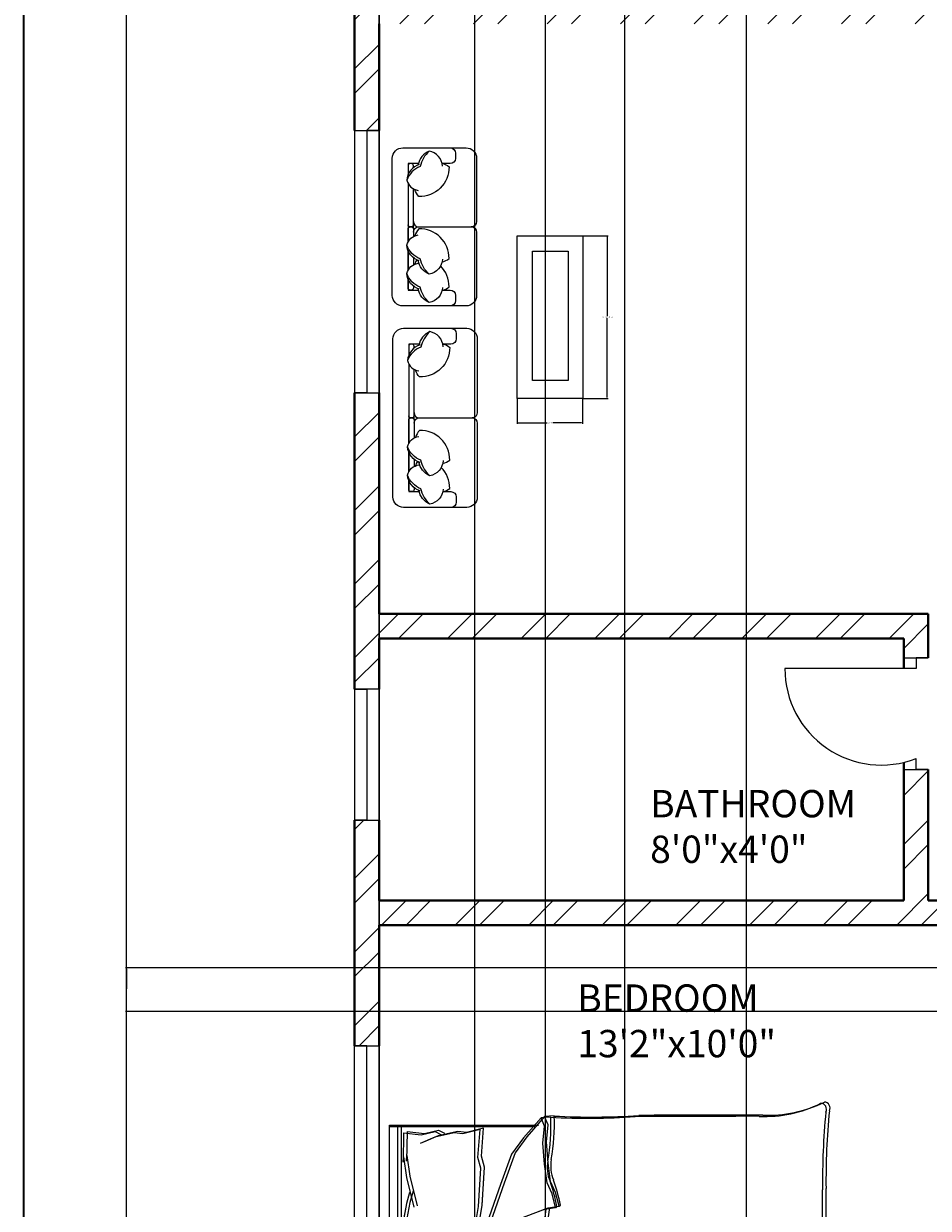
# Model space of a CAD drawing. Units: inches. Extents: x 2063 to 2617, y 1299 to 2210.
# Tile 2 of 22: x 2063 to 2228, y 1510 to 1727. Entities that reach past the tile are written whole.
import ezdxf

# ---------------------------------------------------------------- set-up
doc = ezdxf.new("R2010")
doc.units = ezdxf.units.IN
for name, color, linetype, lineweight in [('A-ANNO-DIMS', 2, 'Continuous', 18), ('A-ANNO-TTLB', 7, 'Continuous', 35), ('A-AREA-IDEN', 7, 'Continuous', 18), ('A-DOOR', 11, 'Continuous', 25), ('A-FURN', 8, 'Continuous', 18), ('A-GLAZ', 123, 'Continuous', 18), ('A-WALL', 7, 'Continuous', 40)]:
    doc.layers.add(name, color=color, linetype=linetype, lineweight=lineweight)
doc.layers.add('A-WALL-PATT', color=215, linetype='Continuous', lineweight=13, true_color=0xa953a0)
doc.styles.get("Standard").update_dxf_attribs({"font": 'arial.ttf'})
doc.dimstyles.get("Standard").update_dxf_attribs({"dimtxt": 0.18, "dimasz": 0.18, "dimexe": 0.18, "dimexo": 0.0625, "dimgap": 0.09, "dimtad": 0, "dimtih": 1, "dimtoh": 1, "dimdec": 4, "dimzin": 0, "dimdsep": 46, "dimtxsty": 'Standard', "dimcen": 0.09, "dimadec": 0, "dimazin": 0, "dimtfac": 1, "dimtdec": 4, "dimtofl": 0, "dimtmove": 0, "dimatfit": 3, "dimfxl": 1, "dimtolj": 1, "dimtzin": 0, "dimarcsym": 0})

# ---------------------------------------------------------------- blocks, each defined once
blk = doc.blocks.new('BED-DOUBLE')
for p, q in [((3.48, 63.33), (3.48, 81.44)), ((3.48, 63.33), (3.48, 81.44)), ((3.48, 81.44), (51.49, 81.44)), ((3.7, 62.69), (3.7, 80.8)), ((3.7, 62.69), (3.7, 80.8)), ((51.27, 81.44), (51.27, 54.83)), ((51.27, 81.44), (51.27, 54.83)), ((51.49, 81.44), (51.49, 80.8)), ((51.49, 80.8), (51.49, 54.19)), ((51.49, 80.8), (51.49, 54.19)), ((3.48, 79.91), (51.27, 79.91)), ((3.48, 79.91), (51.27, 79.91)), ((3.7, 79.27), (51.49, 79.27)), ((3.7, 79.27), (51.49, 79.27)), ((3.89, 78.13), (4.47, 74.95)), ((3.9, 78.11), (8.18, 78.43)), ((3.9, 78.11), (8.18, 78.43)), ((3.9, 78.13), (4.47, 74.95)), ((8.18, 78.43), (8.29, 78.42)), ((8.18, 78.43), (8.29, 78.42)), ((8.29, 78.42), (12.11, 78.13)), ((8.29, 78.42), (12.11, 78.13)), ((12.11, 78.13), (17.6, 77.12)), ((12.11, 78.13), (17.6, 77.12)), ((14.86, 77.69), (16.88, 78.42)), ((14.86, 77.69), (16.88, 78.42)), ((16.88, 78.42), (19.77, 79.14)), ((16.88, 78.42), (19.77, 79.14)), ((17.11, 77.78), (20, 78.5)), ((17.11, 77.78), (20, 78.5)), ((19.77, 79.14), (20.09, 79.14)), ((19.77, 79.14), (20.09, 79.14)), ((20, 78.5), (20.32, 78.5)), ((20, 78.5), (20.32, 78.5)), ((20.09, 79.14), (24.54, 79)), ((20.09, 79.14), (24.54, 79)), ((20.32, 78.5), (24.77, 78.36)), ((20.32, 78.5), (24.77, 78.36)), ((24.54, 79), (25.98, 79.57)), ((24.54, 79), (25.98, 79.57)), ((24.77, 78.36), (26.21, 78.93)), ((24.77, 78.36), (26.21, 78.93)), ((25.98, 79.57), (26.56, 74.22)), ((25.98, 79.57), (26.56, 74.22)), ((26.21, 78.93), (26.79, 73.58)), ((26.21, 78.93), (26.79, 73.58)), ((27.98, 78.95), (27.73, 73.58)), ((27.98, 78.95), (27.73, 73.58)), ((28.21, 78.31), (27.96, 72.94)), ((28.21, 78.31), (27.96, 72.94)), ((29.46, 78.46), (27.98, 78.95)), ((29.46, 78.46), (27.98, 78.95)), ((29.68, 77.83), (28.21, 78.31)), ((29.68, 77.83), (28.21, 78.31)), ((33.88, 78.89), (29.46, 78.46)), ((33.88, 78.89), (29.46, 78.46)), ((34.11, 78.25), (29.68, 77.83)), ((34.11, 78.25), (29.68, 77.83)), ((34.21, 78.91), (33.88, 78.89)), ((34.2, 78.91), (33.88, 78.89)), ((34.43, 78.27), (34.11, 78.25)), ((34.43, 78.27), (34.11, 78.25)), ((37.14, 78.37), (34.2, 78.91)), ((37.14, 78.37), (34.21, 78.91)), ((37.36, 77.73), (34.43, 78.27)), ((37.36, 77.73), (34.43, 78.27)), ((41.91, 78.37), (36.5, 77.02)), ((41.91, 78.37), (36.5, 77.02)), ((39.2, 77.77), (37.14, 78.37)), ((39.2, 77.77), (37.14, 78.37)), ((45.71, 78.9), (41.91, 78.37)), ((45.71, 78.9), (41.91, 78.37)), ((45.94, 78.26), (42.14, 77.73)), ((45.94, 78.26), (42.14, 77.73)), ((50.11, 78.89), (44.71, 78.98)), ((44.71, 78.98), (45.71, 78.9)), ((50.11, 78.89), (44.71, 78.98)), ((44.71, 78.98), (45.71, 78.9)), ((50.34, 78.25), (44.94, 78.34)), ((44.94, 78.34), (45.94, 78.26)), ((50.34, 78.25), (44.94, 78.34)), ((44.94, 78.34), (45.94, 78.26)), ((50.11, 78.89), (49.73, 75.68)), ((50.11, 78.89), (49.73, 75.68)), ((50.34, 78.25), (49.96, 75.04)), ((50.34, 78.25), (49.96, 75.04)), ((4.12, 77.49), (4.7, 74.31)), ((4.12, 77.49), (4.7, 74.31)), ((4.13, 77.47), (8.41, 77.8)), ((4.13, 77.47), (8.41, 77.8)), ((8.41, 77.8), (8.51, 77.78)), ((8.41, 77.8), (8.51, 77.78)), ((8.51, 77.78), (12.34, 77.49)), ((8.51, 77.78), (12.34, 77.49)), ((12.34, 77.49), (17.83, 76.48)), ((12.34, 77.49), (17.83, 76.48)), ((15.08, 77.05), (17.11, 77.78)), ((15.08, 77.05), (17.11, 77.78)), ((42.14, 77.73), (36.72, 76.38)), ((42.14, 77.73), (36.72, 76.38)), ((39.43, 77.13), (37.36, 77.73)), ((39.43, 77.13), (37.36, 77.73)), ((4.47, 74.95), (4.04, 72.34)), ((4.47, 74.95), (4.04, 72.34)), ((4.7, 74.31), (4.27, 71.7)), ((4.7, 74.31), (4.27, 71.7)), ((5.05, 72.49), (6.06, 75.24)), ((5.05, 72.49), (6.06, 75.24)), ((5.28, 71.85), (6.29, 74.6)), ((5.28, 71.85), (6.29, 74.6)), ((26.56, 74.22), (27.14, 71.04)), ((26.56, 74.22), (27.14, 71.04)), ((49.31, 73.19), (48.13, 75.87)), ((49.31, 73.19), (48.13, 75.87)), ((49.54, 72.55), (48.36, 75.23)), ((49.54, 72.55), (48.36, 75.23)), ((49.73, 75.68), (50.33, 73.11)), ((49.73, 75.68), (50.33, 73.11)), ((49.96, 75.04), (50.56, 72.47)), ((49.96, 75.04), (50.56, 72.47)), ((4.04, 72.34), (4.62, 71.33)), ((4.04, 72.34), (4.62, 71.33)), ((4.27, 71.7), (4.85, 70.69)), ((4.27, 71.7), (4.85, 70.69)), ((4.47, 68.87), (5.05, 72.49)), ((4.47, 68.87), (5.05, 72.49)), ((4.7, 68.23), (5.28, 71.85)), ((4.7, 68.23), (5.28, 71.85)), ((26.79, 73.58), (27.37, 70.4)), ((26.79, 73.58), (27.37, 70.4)), ((27.73, 73.58), (27.36, 70.37)), ((27.73, 73.58), (27.36, 70.37)), ((27.96, 72.94), (27.58, 69.73)), ((27.96, 72.94), (27.58, 69.73)), ((50.11, 69.61), (49.31, 73.19)), ((50.11, 69.61), (49.31, 73.19)), ((50.34, 68.98), (49.54, 72.55)), ((50.34, 68.98), (49.54, 72.55)), ((50.33, 73.11), (49.81, 72.06)), ((50.33, 73.11), (49.82, 72.06)), ((50.56, 72.47), (50.04, 71.42)), ((50.56, 72.47), (50.04, 71.42)), ((27.14, 69.74), (26.56, 67.86)), ((27.14, 69.74), (26.56, 67.86)), ((27.14, 71.04), (27.14, 69.74)), ((27.14, 71.04), (27.14, 69.74)), ((27.36, 70.37), (27.44, 69.07)), ((27.36, 70.37), (27.44, 69.07)), ((27.37, 70.4), (27.37, 69.1)), ((27.37, 70.4), (27.37, 69.1)), ((27.58, 69.73), (27.66, 68.43)), ((27.58, 69.73), (27.66, 68.43)), ((49.92, 68.01), (50.11, 69.61)), ((49.92, 68.01), (50.11, 69.61)), ((4.18, 64.1), (4.76, 67.28)), ((4.18, 64.1), (4.76, 67.28)), ((4.76, 67.28), (4.47, 68.87)), ((4.76, 67.28), (4.47, 68.87)), ((4.99, 66.64), (4.7, 68.23)), ((4.99, 66.64), (4.7, 68.23)), ((26.56, 67.86), (26.56, 65.18)), ((26.56, 67.86), (26.56, 65.18)), ((27.37, 69.1), (26.79, 67.22)), ((27.37, 69.1), (26.79, 67.22)), ((26.79, 67.22), (26.79, 64.54)), ((26.79, 67.22), (26.79, 64.54)), ((27.44, 69.07), (28.13, 67.23)), ((27.44, 69.07), (28.13, 67.23)), ((27.66, 68.43), (28.36, 66.59)), ((27.66, 68.43), (28.36, 66.59)), ((28.13, 67.23), (28.3, 64.55)), ((28.13, 67.23), (28.3, 64.55)), ((50.7, 64.87), (49.92, 68.01)), ((50.7, 64.87), (49.92, 68.01)), ((50.15, 67.37), (50.34, 68.98)), ((50.15, 67.37), (50.34, 68.98)), ((50.93, 64.23), (50.15, 67.37)), ((50.93, 64.23), (50.15, 67.37)), ((4.41, 63.46), (4.99, 66.64)), ((4.41, 63.46), (4.99, 66.64)), ((6.38, 65.82), (10.41, 65.15)), ((6.38, 65.82), (10.41, 65.15)), ((6.61, 65.18), (10.64, 64.51)), ((6.61, 65.18), (10.64, 64.51)), ((10.41, 65.15), (9.28, 64.83)), ((10.41, 65.15), (9.28, 64.83)), ((10.41, 65.15), (17.42, 64.72)), ((10.41, 65.15), (17.42, 64.72)), ((17.42, 64.72), (19.38, 65.27)), ((17.42, 64.72), (19.38, 65.27)), ((19.38, 65.27), (24.52, 64.87)), ((19.38, 65.27), (24.52, 64.87)), ((24.1, 65.18), (20.96, 66.27)), ((24.1, 65.18), (20.96, 66.27)), ((24.33, 64.54), (21.19, 65.63)), ((24.33, 64.54), (21.19, 65.63)), ((26.56, 65.18), (24.1, 65.18)), ((26.56, 65.18), (24.1, 65.18)), ((28.36, 66.59), (28.53, 63.91)), ((28.36, 66.59), (28.53, 63.91)), ((30.75, 64.7), (33.82, 65.99)), ((30.75, 64.7), (33.82, 65.99)), ((30.98, 64.06), (34.05, 65.35)), ((30.98, 64.06), (34.05, 65.35)), ((32.56, 65.82), (36.6, 65.15)), ((32.56, 65.82), (36.6, 65.15)), ((32.79, 65.18), (36.83, 64.51)), ((32.79, 65.18), (36.82, 64.51)), ((36.6, 65.15), (43.61, 64.72)), ((36.6, 65.15), (43.61, 64.72)), ((43.61, 64.72), (45.57, 65.27)), ((43.61, 64.72), (45.57, 65.27)), ((45.57, 65.27), (50.7, 64.87)), ((45.57, 65.27), (50.7, 64.87)), ((9.28, 64.83), (4.18, 64.1)), ((9.28, 64.83), (4.18, 64.1)), ((9.51, 64.19), (4.41, 63.46)), ((9.51, 64.19), (4.41, 63.46)), ((10.64, 64.51), (9.51, 64.19)), ((10.64, 64.51), (9.51, 64.19)), ((10.64, 64.51), (17.65, 64.08)), ((10.64, 64.51), (17.65, 64.08)), ((17.65, 64.08), (19.61, 64.64)), ((17.65, 64.08), (19.61, 64.64)), ((19.61, 64.64), (24.74, 64.23)), ((19.61, 64.64), (24.74, 64.23)), ((26.79, 64.54), (24.33, 64.54)), ((26.79, 64.54), (24.33, 64.54)), ((28.3, 64.55), (30.75, 64.7)), ((28.3, 64.55), (30.75, 64.7)), ((28.53, 63.91), (30.98, 64.06)), ((28.53, 63.91), (30.98, 64.06)), ((30.26, 64.06), (34.45, 57.57)), ((30.26, 64.06), (34.45, 57.57)), ((30.49, 63.42), (34.68, 56.93)), ((30.49, 63.42), (34.68, 56.93)), ((40.64, 61.13), (32.31, 64.06)), ((40.64, 61.13), (32.31, 64.06)), ((40.87, 60.49), (32.53, 63.42)), ((40.87, 60.49), (32.54, 63.42)), ((36.82, 64.51), (43.83, 64.08)), ((36.83, 64.51), (43.84, 64.08)), ((43.83, 64.08), (45.8, 64.64)), ((43.84, 64.08), (45.8, 64.64)), ((45.8, 64.64), (50.93, 64.23)), ((45.8, 64.64), (50.93, 64.23)), ((46.22, 59.11), (40.64, 61.13)), ((46.22, 59.11), (40.64, 61.13)), ((46.45, 58.48), (40.87, 60.49)), ((46.45, 58.48), (40.87, 60.49)), ((49.16, 56.95), (46.22, 59.11)), ((49.16, 56.95), (46.22, 59.11)), ((34.45, 57.57), (36.15, 53.08)), ((34.45, 57.57), (36.15, 53.08)), ((34.68, 56.93), (36.38, 52.44)), ((34.68, 56.93), (36.38, 52.44)), ((49.39, 56.31), (46.45, 58.48)), ((49.39, 56.31), (46.45, 58.48)), ((52.87, 53.7), (49.16, 56.95)), ((52.87, 53.7), (49.16, 56.95)), ((53.1, 53.06), (49.39, 56.31)), ((53.1, 53.06), (49.39, 56.31)), ((36.15, 53.08), (36.46, 51.07)), ((36.15, 53.08), (36.46, 51.07)), ((36.38, 52.44), (36.69, 50.43)), ((36.38, 52.44), (36.69, 50.43)), ((38.94, 51.69), (40.95, 52.61)), ((38.94, 51.69), (40.95, 52.61)), ((40.95, 52.61), (44.36, 53.08)), ((40.95, 52.61), (44.36, 53.08)), ((41.18, 51.97), (44.59, 52.44)), ((41.18, 51.97), (44.59, 52.44)), ((44.36, 53.08), (48.23, 53.39)), ((44.36, 53.08), (48.23, 53.39)), ((44.59, 52.44), (48.46, 52.75)), ((44.59, 52.44), (48.46, 52.75)), ((48.23, 53.39), (51.33, 53.08)), ((48.23, 53.39), (51.33, 53.08)), ((48.46, 52.75), (51.56, 52.44)), ((48.46, 52.75), (51.56, 52.44)), ((51.33, 53.08), (52.87, 53.7)), ((51.33, 53.08), (52.87, 53.7)), ((51.56, 52.44), (53.1, 53.06)), ((51.56, 52.44), (53.1, 53.06)), ((52.95, 51.95), (52.87, 53.7, 3.87)), ((52.95, 51.95), (52.87, 53.7, 3.87)), ((53.18, 51.31), (53.1, 53.06, 3.87)), ((53.18, 51.31), (53.1, 53.06, 3.87)), ((36.46, 51.07), (38.94, 51.69)), ((36.46, 51.07), (38.94, 51.69)), ((36.69, 50.43), (39.17, 51.05)), ((36.69, 50.43), (39.17, 51.05)), ((39.17, 51.05), (41.18, 51.97)), ((39.17, 51.05), (41.18, 51.97)), ((15.06, 2.2), (39.68, 2.2)), ((15.06, 2.2), (39.68, 2.2)), ((15.29, 1.56), (39.91, 1.56)), ((15.29, 1.56), (39.91, 1.56))]:
    blk.add_line(p, q)
for centre, radius, start, end in [((85.16, 61.35), 83.31, 178.7218, 185.604), ((85.16, 61.35), 83.31, 178.7218, 185.604), ((21.36, -100.61), 164.97, 86.0865, 96.7821), ((21.36, -100.61), 164.97, 86.0865, 96.7821), ((21.59, -101.25), 164.97, 86.0865, 96.7821), ((21.59, -101.25), 164.97, 86.0865, 96.7821), ((85.39, 60.71), 83.31, 178.7218, 185.604), ((85.39, 60.71), 83.31, 178.7218, 185.604), ((17.76, -74.87), 129.02, 81.7845, 96.9006), ((17.76, -74.87), 129.02, 81.7845, 96.9006), ((17.98, -75.51), 129.02, 81.7845, 96.9006), ((17.98, -75.51), 129.02, 81.7845, 96.9006), ((-167.31, 50.27), 170.11, 358.4762, 1.0082), ((-167.31, 50.27), 170.11, 358.4762, 1.0082), ((-167.08, 49.63), 170.11, 358.4762, 1.0082), ((-167.08, 49.63), 170.11, 358.4762, 1.0082), ((31.15, 79.96), 29.65, 280.6617, 289.8806), ((31.15, 79.96), 29.65, 280.6617, 289.8806), ((43.74, 46.38), 6.22, 78.6608, 113.7384), ((43.74, 46.38), 6.22, 78.6608, 113.7384), ((51.33, 88.1), 36.18, 259.8763, 272.5657), ((51.33, 88.1), 36.18, 259.8763, 272.5657), ((36.64, 51), 0.185, 160.2464, 271.1377), ((36.64, 51), 0.185, 160.2464, 271.1377), ((36.87, 50.36), 0.185, 160.2464, 271.1377), ((36.86, 50.36), 0.185, 160.2464, 271.1377), ((31.38, 79.32), 29.65, 280.6617, 289.8806), ((31.38, 79.32), 29.65, 280.6617, 289.8806), ((43.97, 45.74), 6.22, 78.6608, 113.7384), ((43.97, 45.74), 6.22, 78.6608, 113.7384), ((51.56, 87.46), 36.18, 259.8763, 272.5657), ((51.56, 87.46), 36.18, 259.8763, 272.5657), ((182.27, 45.13), 129.5, 176.9791, 183.8365), ((182.27, 45.13), 129.5, 176.9791, 183.8365), ((182.49, 44.49), 129.5, 176.9791, 183.8365), ((182.49, 44.49), 129.5, 176.9791, 183.8365), ((484.82, 30.83), 482.31, 178.2277, 181.7185), ((484.82, 30.83), 482.31, 178.2277, 181.7185), ((485.05, 30.19), 482.31, 178.2277, 181.7185), ((485.05, 30.19), 482.31, 178.2277, 181.7185), ((-4508.74, 13.62), 4561.86, 0.00217, 0.28689), ((-4508.74, 13.62), 4561.86, 0.00217, 0.28689), ((-4508.51, 12.98), 4561.86, 0.00217, 0.28689), ((-4508.51, 12.98), 4561.86, 0.00217, 0.28689), ((-26.9, 16.93), 29.63, 346.0648, 358.9113), ((-26.9, 16.93), 29.63, 346.0648, 358.9113), ((-26.67, 16.29), 29.63, 346.0648, 358.9113), ((-26.67, 16.29), 29.63, 346.0648, 358.9113), ((76.16, 12.78), 23.07, 177.4714, 206.4681), ((76.16, 12.78), 23.07, 177.4714, 206.4681), ((76.39, 12.14), 23.07, 177.4714, 206.4681), ((76.39, 12.14), 23.07, 177.4714, 206.4681), ((-21.66, 11.17), 23.56, 337.9751, 356.652), ((-21.66, 11.17), 23.56, 337.9751, 356.652), ((-21.43, 10.53), 23.56, 337.9751, 356.652), ((-21.43, 10.53), 23.56, 337.9751, 356.652), ((1.09, 1.73), 1.09, 146.1736, 293.4781), ((1.09, 1.73), 1.09, 146.1736, 293.4781), ((21.43, -119.39), 121.76, 92.9958, 99.4091), ((21.43, -119.39), 121.76, 92.9958, 99.4091), ((-17.22, 105.16), 106.46, 283.3832, 287.7053), ((-17.22, 105.16), 106.46, 283.3832, 287.7053), ((-16.99, 104.52), 106.46, 283.3832, 287.7053), ((-16.99, 104.52), 106.46, 283.3832, 287.7053), ((41.15, -130.83), 133.04, 84.4998, 90.6351), ((41.15, -130.83), 133.04, 84.4998, 90.6351), ((54.41, 2.57), 1.1, 242.6588, 356.02), ((54.41, 2.57), 1.1, 242.6588, 356.02), ((1.32, 1.09), 1.09, 146.1736, 293.4781), ((1.32, 1.09), 1.09, 146.1736, 293.4781), ((21.66, -120.03), 121.76, 92.9958, 99.4091), ((21.66, -120.03), 121.76, 92.9958, 99.4091), ((41.38, -131.47), 133.04, 84.4998, 90.6351), ((41.38, -131.47), 133.04, 84.4998, 90.6351), ((54.64, 1.93), 1.1, 242.6588, 356.02), ((54.64, 1.93), 1.1, 242.6588, 356.02)]:
    blk.add_arc(centre, radius, start, end)
blk = doc.blocks.new('WIN-60IN')
for p, q in [((0, 60), (4.5, 60)), ((0, 60), (0, 0)), ((4.5, 60), (2.25, 60)), ((2.25, 60), (2.25, 0)), ((4.5, 60), (4.5, 0)), ((2.25, 0), (0, 0)), ((0, 0), (4.5, 0))]:
    blk.add_line(p, q)
blk = doc.blocks.new('TABLE-COFFEE')
for points in [[(0, 29.74), (11.98, 29.74), (11.98, 0), (0, 0)], [(2.66, 26.46), (2.66, 26.46), (2.66, 26.46), (2.66, 26.46)], [(2.66, 26.46), (2.66, 26.46), (2.66, 26.46), (2.66, 26.46)], [(2.66, 26.46), (2.66, 26.46), (2.66, 26.46), (2.66, 26.46)], [(2.66, 26.46), (9.18, 26.46), (9.18, 2.77), (2.66, 2.77)]]:
    blk.add_lwpolyline(points, close=True)
blk = doc.blocks.new('*D29')
at = {"layer": 'A-ANNO-DIMS', "color": 0, "lineweight": -2, "transparency": 16777216}
for p, q in [((2164.95, 1688.47), (2169.53, 1688.47)), ((2169.35, 1688.29), (2169.35, 1673.78)), ((2169.35, 1658.91), (2169.35, 1673.42)), ((2164.95, 1658.73), (2169.53, 1658.73))]:
    blk.add_line(p, q, dxfattribs=at)
at = {"layer": 'A-ANNO-DIMS', "color": 0, "transparency": 16777216}
for points in [[(2169.32, 1688.29), (2169.38, 1688.29), (2169.35, 1688.47)], [(2169.32, 1658.91), (2169.38, 1658.91), (2169.35, 1658.73)]]:
    blk.add_solid(points, dxfattribs=at)
at = {"layer": 'Defpoints', "color": 0, "transparency": 16777216}
for p in [(2164.88, 1688.47), (2164.88, 1658.73), (2169.35, 1658.73)]:
    blk.add_point(p, dxfattribs=at)
at = {"layer": 'A-ANNO-DIMS', "color": 0, "transparency": 16777216, "insert": (2169.35, 1673.6), "char_height": 0.18, "attachment_point": 5}
blk.add_mtext('\\A1;LOW TABLE 30 TYP.', dxfattribs=at)
blk = doc.blocks.new('*D30')
at = {"layer": 'A-ANNO-DIMS', "color": 0, "lineweight": -2, "transparency": 16777216}
for p, q in [((2152.9, 1658.67), (2152.9, 1654.09)), ((2164.88, 1658.67), (2164.88, 1654.09)), ((2153.08, 1654.27), (2158.37, 1654.27)), ((2164.7, 1654.27), (2159.41, 1654.27))]:
    blk.add_line(p, q, dxfattribs=at)
at = {"layer": 'A-ANNO-DIMS', "color": 0, "transparency": 16777216}
for points in [[(2153.08, 1654.3), (2153.08, 1654.24), (2152.9, 1654.27)], [(2164.7, 1654.3), (2164.7, 1654.24), (2164.88, 1654.27)]]:
    blk.add_solid(points, dxfattribs=at)
at = {"layer": 'Defpoints', "color": 0, "transparency": 16777216}
for p in [(2152.9, 1658.73), (2164.88, 1658.73), (2152.9, 1654.27)]:
    blk.add_point(p, dxfattribs=at)
at = {"layer": 'A-ANNO-DIMS', "color": 0, "transparency": 16777216, "insert": (2158.89, 1654.27), "char_height": 0.18, "attachment_point": 5}
blk.add_mtext('\\A1;12 TYP.', dxfattribs=at)
blk = doc.blocks.new('*D32')
at = {"layer": 'A-ANNO-DIMS', "color": 0, "lineweight": -2, "transparency": 16777216}
for p, q in [((2123.08, 2128.81), (2081.21, 2128.81)), ((2081.39, 2128.63), (2081.39, 1765.49)), ((2081.39, 1401.99), (2081.39, 1765.13)), ((2123.08, 1401.81), (2081.21, 1401.81))]:
    blk.add_line(p, q, dxfattribs=at)
at = {"layer": 'A-ANNO-DIMS', "color": 0, "transparency": 16777216}
for points in [[(2081.36, 2128.63), (2081.42, 2128.63), (2081.39, 2128.81)], [(2081.36, 1401.99), (2081.42, 1401.99), (2081.39, 1401.81)]]:
    blk.add_solid(points, dxfattribs=at)
at = {"layer": 'Defpoints', "color": 0, "transparency": 16777216}
for p in [(2081.39, 2128.81), (2123.14, 2128.81), (2123.14, 1401.81)]:
    blk.add_point(p, dxfattribs=at)
at = {"layer": 'A-ANNO-DIMS', "color": 0, "transparency": 16777216, "insert": (2081.39, 1765.31), "char_height": 0.18, "attachment_point": 5}
blk.add_mtext('\\A1;727', dxfattribs=at)
blk = doc.blocks.new('*D49')
at = {"layer": 'A-ANNO-DIMS', "color": 0, "lineweight": -2, "transparency": 16777216}
for p, q in [((2127.64, 2124.25), (2127.64, 1317.7)), ((2158.04, 2124.25), (2158.04, 1317.7)), ((2127.82, 1317.88), (2142.38, 1317.88)), ((2157.86, 1317.88), (2143.31, 1317.88))]:
    blk.add_line(p, q, dxfattribs=at)
at = {"layer": 'A-ANNO-DIMS', "color": 0, "transparency": 16777216}
for points in [[(2127.82, 1317.91), (2127.82, 1317.85), (2127.64, 1317.88)], [(2157.86, 1317.91), (2157.86, 1317.85), (2158.04, 1317.88)]]:
    blk.add_solid(points, dxfattribs=at)
at = {"layer": 'Defpoints', "color": 0, "transparency": 16777216}
for p in [(2127.64, 2124.31), (2158.04, 2124.31), (2158.04, 1317.88)]:
    blk.add_point(p, dxfattribs=at)
at = {"layer": 'A-ANNO-DIMS', "color": 0, "transparency": 16777216, "insert": (2142.84, 1317.88), "char_height": 0.18, "attachment_point": 5}
blk.add_mtext('\\A1;30.396', dxfattribs=at)
blk = doc.blocks.new('*D57')
at = {"layer": 'A-ANNO-DIMS', "color": 0, "lineweight": -2, "transparency": 16777216}
for p, q in [((2172.52, 1868.25), (2172.52, 1317.7)), ((2194.82, 1868.25), (2194.82, 1317.7)), ((2172.7, 1317.88), (2183.2, 1317.88)), ((2194.64, 1317.88), (2184.14, 1317.88))]:
    blk.add_line(p, q, dxfattribs=at)
at = {"layer": 'A-ANNO-DIMS', "color": 0, "transparency": 16777216}
for points in [[(2172.7, 1317.91), (2172.7, 1317.85), (2172.52, 1317.88)], [(2194.64, 1317.91), (2194.64, 1317.85), (2194.82, 1317.88)]]:
    blk.add_solid(points, dxfattribs=at)
at = {"layer": 'Defpoints', "color": 0, "transparency": 16777216}
for p in [(2172.52, 1868.31), (2194.82, 1868.31), (2194.82, 1317.88)]:
    blk.add_point(p, dxfattribs=at)
at = {"layer": 'A-ANNO-DIMS', "color": 0, "transparency": 16777216, "insert": (2183.67, 1317.88), "char_height": 0.18, "attachment_point": 5}
blk.add_mtext('\\A1;22.305', dxfattribs=at)
blk = doc.blocks.new('*D58')
at = {"layer": 'A-ANNO-DIMS', "color": 0, "lineweight": -2, "transparency": 16777216}
for p, q in [((2290.08, 1554.5), (2081.21, 1554.5)), ((2081.39, 1554.32), (2081.39, 1550.68)), ((2081.39, 1546.68), (2081.39, 1550.32)), ((2290.08, 1546.5), (2081.21, 1546.5))]:
    blk.add_line(p, q, dxfattribs=at)
at = {"layer": 'A-ANNO-DIMS', "color": 0, "transparency": 16777216}
for points in [[(2081.36, 1554.32), (2081.42, 1554.32), (2081.39, 1554.5)], [(2081.36, 1546.68), (2081.42, 1546.68), (2081.39, 1546.5)]]:
    blk.add_solid(points, dxfattribs=at)
at = {"layer": 'Defpoints', "color": 0, "transparency": 16777216}
for p in [(2081.39, 1554.5), (2290.14, 1554.5), (2290.14, 1546.5)]:
    blk.add_point(p, dxfattribs=at)
at = {"layer": 'A-ANNO-DIMS', "color": 0, "transparency": 16777216, "insert": (2081.39, 1550.5), "char_height": 0.18, "attachment_point": 5}
blk.add_mtext('\\A1;8', dxfattribs=at)
blk = doc.blocks.new('*D61')
at = {"layer": 'A-ANNO-DIMS', "color": 0, "lineweight": -2, "transparency": 16777216}
for p, q in [((2127.64, 1442.37), (2127.64, 2170.74)), ((2127.82, 2170.56), (2136.03, 2170.56)), ((2144.97, 2170.56), (2136.77, 2170.56)), ((2145.15, 1442.37), (2145.15, 2170.74))]:
    blk.add_line(p, q, dxfattribs=at)
at = {"layer": 'A-ANNO-DIMS', "color": 0, "transparency": 16777216}
for points in [[(2127.82, 2170.59), (2127.82, 2170.53), (2127.64, 2170.56)], [(2144.97, 2170.59), (2144.97, 2170.53), (2145.15, 2170.56)]]:
    blk.add_solid(points, dxfattribs=at)
at = {"layer": 'Defpoints', "color": 0, "transparency": 16777216}
for p in [(2145.15, 2170.56), (2127.64, 1442.31), (2145.15, 1442.31)]:
    blk.add_point(p, dxfattribs=at)
at = {"layer": 'A-ANNO-DIMS', "color": 0, "transparency": 16777216, "insert": (2136.4, 2170.56), "char_height": 0.18, "attachment_point": 5}
blk.add_mtext('\\A1;17.51', dxfattribs=at)

msp = doc.modelspace()

# ---------------------------------------------------------------- hatches: boundary and pattern name
at = {"layer": 'A-WALL-PATT'}
h = msp.add_hatch(dxfattribs=at)
h.set_pattern_fill('ANSI32', color=256)
h.paths.add_polyline_path([(2553.6442, 2128.8122), (2511.1703, 2128.8122), (2511.1703, 2124.3122), (2549.1442, 2124.3122), (2549.1442, 2095.662), (2553.6442, 2095.662)])
h.paths.add_polyline_path([(2553.6442, 2035.662), (2549.1442, 2035.662), (2549.1442, 1980.3122), (2503.7214, 1980.3122), (2503.7214, 1975.8122), (2549.1442, 1975.8122), (2549.1442, 1962.9693), (2553.6442, 1962.9693)])
h.paths.add_polyline_path([(2553.6442, 1938.9693), (2549.1442, 1938.9693), (2549.1442, 1927.8122), (2477.1442, 1927.8122), (2477.1442, 1975.8122), (2481.2918, 1975.8122), (2481.2918, 1980.3122), (2453.2648, 1980.3122), (2453.2648, 1975.8122), (2472.6442, 1975.8122), (2472.6442, 1868.3122), (2400.6442, 1868.3122), (2400.6442, 1861.3782), (2405.1442, 1861.3782), (2405.1442, 1863.8122), (2480.9699, 1863.8122), (2480.9699, 1866.0622), (2480.9699, 1868.3122), (2477.1442, 1868.3122), (2477.1442, 1923.3122), (2549.1442, 1923.3122), (2549.1442, 1908.8504), (2553.6442, 1908.8504)])
h.paths.add_polyline_path([(2553.6442, 1884.8504), (2549.1442, 1884.8504), (2549.1442, 1868.3122), (2501.0636, 1868.3122), (2501.0636, 1863.8122), (2549.1442, 1863.8122), (2549.1442, 1826.0298), (2553.6442, 1826.0298)])
h.paths.add_polyline_path([(2388.1504, 1980.3122), (2340.6442, 1980.3122), (2340.6442, 2124.3122), (2358.7501, 2124.3122), (2358.7501, 2128.8122), (2316.3482, 2128.8122), (2316.3482, 2124.3122), (2336.1442, 2124.3122), (2336.1442, 1980.3122), (2289.1737, 1980.3122), (2289.1737, 1975.8122), (2336.1442, 1975.8122), (2336.1442, 1619.3122), (2333.1433, 1619.3122), (2333.1433, 1614.8122), (2344.1671, 1614.8122), (2344.1671, 1617.0622), (2344.1671, 1619.3122), (2340.6442, 1619.3122), (2340.6442, 1975.8122), (2388.1504, 1975.8122), (2388.1504, 1978.0622)])
h.paths.add_polyline_path([(2290.1442, 1614.8122), (2301.4594, 1614.8122), (2301.4594, 1617.0622), (2301.4594, 1619.3122), (2285.6442, 1619.3122), (2285.6442, 1566.8122), (2280.8619, 1566.8122), (2280.8619, 1564.5622), (2280.8619, 1562.3122), (2285.6442, 1562.3122), (2285.6442, 1442.3122), (2281.7879, 1442.3122), (2281.7879, 1437.8122), (2285.6442, 1437.8122), (2285.6442, 1401.8122), (2290.1442, 1401.8122)])
h.paths.add_polyline_path([(2549.1442, 1731.8122), (2405.1442, 1731.8122), (2405.1442, 1834.4638), (2402.8942, 1834.4638), (2400.6442, 1834.4638), (2400.6442, 1727.3122), (2549.1442, 1727.3122)])
h.paths.add_polyline_path([(2553.6442, 1766.0298), (2551.3942, 1766.0298), (2549.1442, 1766.0298), (2549.1442, 1686.7767), (2553.6442, 1686.7767)])
h.paths.add_polyline_path([(2553.6442, 1638.7767), (2551.3942, 1638.7767), (2549.1442, 1638.7767), (2549.1442, 1619.3122), (2448.6442, 1619.3122), (2448.6442, 1610.5671), (2450.8942, 1610.5671), (2453.1442, 1610.5671), (2453.1442, 1614.8122), (2549.1442, 1614.8122), (2549.1442, 1601.6421), (2553.6442, 1601.6421)])
h.paths.add_polyline_path([(2553.6442, 1577.6421), (2551.3942, 1577.6421), (2549.1442, 1577.6421), (2549.1442, 1566.8122), (2453.1442, 1566.8122), (2453.1442, 1591.5045), (2451.0335, 1591.5045), (2448.6442, 1591.5045), (2448.6442, 1566.8122), (2434.0475, 1566.8122), (2434.0475, 1562.3122), (2549.1442, 1562.3122), (2549.1442, 1533.48), (2553.6442, 1533.48)])
h.paths.add_polyline_path([(2553.6442, 1473.48), (2549.1442, 1473.48), (2549.1442, 1442.3122), (2502.6258, 1442.3122), (2502.6258, 1437.8122), (2549.1442, 1437.8122), (2549.1442, 1401.8122), (2553.6442, 1401.8122)])
h.paths.add_polyline_path([(2395.6442, 1562.3122), (2400.0901, 1562.3122), (2400.0901, 1564.5622), (2400.0901, 1566.8122), (2395.6442, 1566.8122), (2395.6442, 1619.3122), (2379.1127, 1619.3122), (2379.1127, 1614.8122), (2391.1442, 1614.8122), (2391.1442, 1401.8122), (2395.6442, 1401.8122), (2395.6442, 1437.8122), (2399.2425, 1437.8122), (2399.2425, 1440.0622), (2399.2425, 1442.3122), (2395.6442, 1442.3122)])
h.paths.add_polyline_path([(2442.6258, 1442.3122), (2419.6262, 1442.3122), (2419.6262, 1437.8122), (2442.6258, 1437.8122), (2442.6258, 1440.0622)])
h.paths.add_polyline_path([(2127.6442, 1480.2532), (2125.3942, 1480.2532), (2123.1442, 1480.2532), (2123.1442, 1401.8122), (2127.6442, 1401.8122), (2127.6442, 1437.8122), (2145.1538, 1437.8122), (2145.1538, 1440.0622), (2145.1538, 1442.3122), (2127.6442, 1442.3122)])
h.paths.add_polyline_path([(2259.809, 1442.3122), (2205.1538, 1442.3122), (2205.1538, 1437.8122), (2259.809, 1437.8122), (2259.809, 1440.0622)])
h.paths.add_polyline_path([(2127.6442, 1659.7652), (2123.1442, 1659.7652), (2123.1442, 1605.5161), (2125.3942, 1605.5161), (2127.6442, 1605.5161), (2127.6442, 1614.8122), (2223.6442, 1614.8122), (2223.6442, 1611.2723), (2228.1442, 1611.2723), (2228.1442, 1619.3122), (2127.6442, 1619.3122)])
h.paths.add_polyline_path([(2244.8673, 1566.8122), (2228.1442, 1566.8122), (2228.1442, 1590.8122), (2225.8942, 1590.8122), (2223.6442, 1590.8122), (2223.6442, 1566.8122), (2127.6442, 1566.8122), (2127.6442, 1581.5161), (2123.1442, 1581.5161), (2123.1442, 1540.2532), (2127.6442, 1540.2532), (2127.6442, 1562.3122), (2244.8673, 1562.3122), (2244.8673, 1564.5622)])
h.paths.add_polyline_path([(2172.5174, 1868.3122), (2127.6442, 1868.3122), (2127.6442, 1886.5833), (2123.1442, 1886.5833), (2123.1442, 1832.6633), (2127.6442, 1832.6633), (2127.6442, 1863.8122), (2172.5174, 1863.8122), (2172.5174, 1866.0622)])
h.paths.add_polyline_path([(2276.1442, 1868.3122), (2204.1442, 1868.3122), (2204.1442, 1923.3122), (2204.1442, 1975.8122), (2224.8362, 1975.8122), (2224.8362, 1978.1097), (2224.8362, 1980.3122), (2195.0729, 1980.3122), (2195.0729, 1978.0622), (2195.0729, 1975.8122), (2199.6442, 1975.8122), (2199.6442, 1927.8122), (2127.6442, 1927.8122), (2127.6442, 1942.3492), (2123.1442, 1942.3492), (2123.1442, 1910.5833), (2127.6442, 1910.5833), (2127.6442, 1923.3122), (2199.6442, 1923.3122), (2199.6442, 1868.3122), (2194.8228, 1868.3122), (2194.8228, 1864.7337), (2194.8228, 1863.8122), (2271.6442, 1863.8122), (2271.6442, 1860.0507), (2276.1442, 1860.0507)])
h.paths.add_polyline_path([(2276.1442, 1829.994), (2273.8942, 1829.994), (2271.6442, 1829.994), (2271.6442, 1731.8122), (2127.6442, 1731.8122), (2127.6442, 1772.6633), (2123.1442, 1772.6633), (2123.1442, 1707.7652), (2127.6442, 1707.7652), (2127.6442, 1727.3122), (2276.1442, 1727.3122)])
h.paths.add_polyline_path([(2127.6442, 2022.1152), (2123.1442, 2022.1152), (2123.1442, 1966.3492), (2127.6442, 1966.3492), (2127.6442, 1975.8122), (2174.2082, 1975.8122), (2174.2082, 1978.0622), (2174.2082, 1980.3122), (2127.6442, 1980.3122)])
h.paths.add_polyline_path([(2361.9755, 1678.588), (2398.4558, 1678.588), (2398.4558, 1697.2453), (2361.9755, 1697.2453)], flags=9)
h.paths.add_polyline_path([(2351.5397, 1780.4072), (2386.1987, 1780.4072), (2386.1987, 1790.7107), (2351.5397, 1790.7107)], flags=25)
h.paths.add_polyline_path([(2350.6753, 1940.9321), (2387.6024, 1940.9321), (2387.6024, 1959.5894), (2350.6753, 1959.5894)], flags=25)
h.paths.add_polyline_path([(2254.9545, 1684.638), (2295.0943, 1684.638), (2295.0943, 1703.2953), (2254.9545, 1703.2953)], flags=9)
h.paths.add_polyline_path([(2282.4946, 1782.4438), (2317.1535, 1782.4438), (2317.1535, 1792.7474), (2282.4946, 1792.7474)], flags=9)
h.paths.add_polyline_path([(2270.327, 1939.2854), (2307.254, 1939.2854), (2307.254, 1957.9428), (2270.327, 1957.9428)], flags=9)

# ---------------------------------------------------------------- linework, layer by layer
at = {"layer": 'A-ANNO-TTLB'}
msp.add_lwpolyline([(2062.5792, 2209.6485), (2617.0648, 2209.6485), (2617.0648, 1299.1125), (2062.5792, 1299.1125)], close=True, dxfattribs=at)
at = {"layer": 'A-DOOR'}
for p, q in [((2223.6442, 1611.2723), (2228.1442, 1611.2723)), ((2228.1442, 1611.2723), (2225.8942, 1611.2723)), ((2225.8942, 1611.2723), (2225.8942, 1609.2723)), ((2225.8942, 1609.2723), (2201.8942, 1609.2723)), ((2225.8942, 1590.8122), (2225.8942, 1592.8122)), ((2223.6442, 1590.8122), (2228.1442, 1590.8122)), ((2228.1442, 1590.8122), (2225.8942, 1590.8122)), ((2228.1442, 1590.8122), (2228.1442, 1590.8122))]:
    msp.add_line(p, q, dxfattribs=at)
msp.add_arc((2219.5387, 1609.2723), 17.6445, 180, 291.112316, dxfattribs=at)
at = {"layer": 'A-FURN', "ltscale": 0.03}
for points in [[(2145.4685, 1691.0922, -0.41421356), (2144.5041, 1690.1278, -0.41421356), (2145.4685, 1689.1634), (2145.4685, 1677.5903, -0.41421356), (2143.5397, 1675.6615), (2131.9666, 1675.6615, -0.41421356), (2130.0377, 1677.5903), (2130.0377, 1702.6653, -0.41421356), (2131.9666, 1704.5942), (2143.5397, 1704.5942, -0.41421356), (2145.4685, 1702.6653), (2145.4685, 1691.0922, -0.41421356), (2144.5041, 1690.1278, -0.41421356), (2145.4685, 1689.1634)], [(2145.5981, 1656.1314, -0.41421356), (2144.6337, 1655.167, -0.41421356), (2145.5981, 1654.2025), (2145.5981, 1640.7006, -0.41421356), (2143.6692, 1638.7718), (2132.0962, 1638.7718, -0.41421356), (2130.1673, 1640.7006), (2130.1673, 1669.6333, -0.41421356), (2132.0962, 1671.5622), (2143.6692, 1671.5622, -0.41421356), (2145.5981, 1669.6333), (2145.5981, 1656.1314, -0.41421356), (2144.6337, 1655.167, -0.41421356), (2145.5981, 1654.2025)]]:
    msp.add_lwpolyline(points, format="xyb", dxfattribs=at)
at = {"layer": 'A-FURN'}
for points in [[(2140.6464, 1704.5942, -0.41421356), (2141.6108, 1703.6297), (2141.6108, 1702.6653, -0.41421356), (2140.6464, 1701.7009), (2139.1522, 1701.7009)], [(2136.7796, 1703.9804, 0.14772988), (2135.1221, 1701.1616, 0.21334276), (2132.6912, 1698.6745, 0.17866181)], [(2139.2105, 1701.2169, 0.35677236), (2136.7796, 1703.9804, 0.24954205), (2134.7763, 1701.4764, -9.61688035)], [(2134.99, 1701.5511, 0.30666349), (2132.6912, 1698.6745, 0.30632997), (2134.7906, 1696.7954, -0.87284716)], [(2133.8954, 1700.9649), (2133.8954, 1701.3151, 0.41421356), (2133.5097, 1701.7009), (2133.3168, 1701.7009, 0.41421356), (2132.931, 1701.3151)], [(2132.931, 1701.3151), (2132.931, 1699.672, 0.41421356)], [(2139.1517, 1701.703, -0.16554063), (2140.426, 1701.1064, -0.42598917), (2134.9011, 1695.69, -0.12152332), (2134.1396, 1696.9757, 7.11546429)], [(2132.931, 1698.0676), (2132.931, 1690.5136, 0.41421356), (2133.3168, 1690.1278), (2133.5097, 1690.1278, 0.41421356), (2133.8954, 1690.5136), (2133.8954, 1697.0964, 0.41421356)], [(2132.931, 1687.3834), (2132.931, 1689.742, -0.41421356), (2133.3168, 1690.1278), (2133.5097, 1690.1278, -0.41421356), (2133.8954, 1689.742), (2133.8954, 1688.3545, -0.41421356)], [(2133.8954, 1691.0922, 0.41421356), (2134.8599, 1690.1278)], [(2133.8954, 1691.0922, 0.41421356), (2134.8599, 1690.1278), (2144.5041, 1690.1278, 0.41421356)], [(2133.8954, 1689.1634, -0.41421356), (2134.8599, 1690.1278)], [(2133.8954, 1689.1634, -0.41421356), (2134.8599, 1690.1278), (2144.5041, 1690.1278, -0.41421356)], [(2139.1517, 1683.7479, 0.16554063), (2140.426, 1684.3446, 0.42598917), (2134.9011, 1689.761, 0.12152332), (2134.1396, 1688.4752, -7.11546429)], [(2134.99, 1683.8999, -0.30666349), (2132.6912, 1686.7764, -0.30632997), (2134.7906, 1688.6556, 0.87284716)], [(2136.7796, 1681.4706, -0.14772988), (2135.1221, 1684.2893, -0.21334276), (2132.6912, 1686.7764, -0.17866181)], [(2132.931, 1682.1881), (2132.931, 1685.7789, -0.41421356)], [(2134.99, 1678.7046, -0.30666349), (2132.6912, 1681.5811, -0.30632997), (2134.7906, 1683.4603, 0.87284716)], [(2133.8954, 1684.486), (2133.8954, 1683.1592, -0.41421356)], [(2134.5167, 1684.0885, 0.07186538), (2134.1396, 1683.2799, -7.11546429)], [(2139.2105, 1684.234, -0.35677236), (2136.7796, 1681.4706, -0.24954205), (2134.7763, 1683.9745, 9.61688035)], [(2139.1517, 1678.5526, 0.16554063), (2140.426, 1679.1493, 0.20023115), (2138.8741, 1682.9777, 0.12152332)], [(2136.7796, 1676.2753, -0.14772988), (2135.1221, 1679.094, -0.21334276), (2132.6912, 1681.5811, -0.17866181)], [(2132.931, 1678.9405), (2132.931, 1680.5836, -0.41421356)], [(2132.931, 1680.5836), (2132.931, 1678.5547), (2134.8263, 1678.5547, -0.41421356)], [(2133.8954, 1679.2907), (2133.8954, 1678.9405, -0.41421356), (2133.5097, 1678.5547), (2133.3168, 1678.5547, -0.41421356), (2132.931, 1678.9405)], [(2139.2105, 1679.0387, -0.35677236), (2136.7796, 1676.2753, -0.24954205), (2134.7763, 1678.7792, 9.61688035)], [(2139.1522, 1678.5547), (2140.6464, 1678.5547, -0.41421356), (2141.6108, 1677.5903), (2141.6108, 1676.6259, -0.41421356), (2140.6464, 1675.6615)], [(2136.9092, 1670.9484, 0.14772988), (2135.2517, 1668.1296, 0.21334276), (2132.8208, 1665.6425, 0.17866181)], [(2139.3401, 1668.1849, 0.35677236), (2136.9092, 1670.9484, 0.24954205), (2134.9058, 1668.4444, -9.61688035)], [(2140.776, 1671.5622, -0.41421356), (2141.7404, 1670.5977), (2141.7404, 1669.6333, -0.41421356), (2140.776, 1668.6689), (2139.2817, 1668.6689)], [(2135.1196, 1668.519, 0.30666349), (2132.8208, 1665.6425, 0.30632997), (2134.9202, 1663.7634, -0.87284716)], [(2134.025, 1667.9329), (2134.025, 1668.2831, 0.41421356), (2133.6392, 1668.6689), (2133.4463, 1668.6689, 0.41421356), (2133.0606, 1668.2831)], [(2133.0606, 1668.2831), (2133.0606, 1666.64, 0.41421356)], [(2139.2813, 1668.671, -0.16554063), (2140.5556, 1668.0744, -0.42598917), (2135.0307, 1662.658, -0.12152332), (2134.2692, 1663.9437, 7.11546429)], [(2133.0606, 1665.0356), (2133.0606, 1655.5527, 0.41421356), (2133.4463, 1655.167), (2133.6392, 1655.167, 0.41421356), (2134.025, 1655.5527), (2134.025, 1664.0644, 0.41421356)], [(2133.0606, 1650.4937), (2133.0606, 1654.7812, -0.41421356), (2133.4463, 1655.167), (2133.6392, 1655.167, -0.41421356), (2134.025, 1654.7812), (2134.025, 1651.4648, -0.41421356)], [(2134.025, 1656.1314, 0.41421356), (2134.9894, 1655.167)], [(2134.025, 1656.1314, 0.41421356), (2134.9894, 1655.167), (2144.6337, 1655.167, 0.41421356)], [(2134.025, 1654.2025, -0.41421356), (2134.9894, 1655.167)], [(2134.025, 1654.2025, -0.41421356), (2134.9894, 1655.167), (2144.6337, 1655.167, -0.41421356)], [(2139.2813, 1646.8582, 0.16554063), (2140.5556, 1647.4549, 0.42598917), (2135.0307, 1652.8713, 0.12152332), (2134.2692, 1651.5855, -7.11546429)], [(2135.1196, 1647.0102, -0.30666349), (2132.8208, 1649.8867, -0.30632997), (2134.9202, 1651.7659, 0.87284716)], [(2136.9092, 1644.5809, -0.14772988), (2135.2517, 1647.3996, -0.21334276), (2132.8208, 1649.8867, -0.17866181)], [(2133.0606, 1645.2984), (2133.0606, 1648.8892, -0.41421356)], [(2135.1196, 1641.8149, -0.30666349), (2132.8208, 1644.6914, -0.30632997), (2134.9202, 1646.5706, 0.87284716)], [(2134.025, 1647.5963), (2134.025, 1646.2695, -0.41421356)], [(2134.6462, 1647.1988, 0.07186538), (2134.2692, 1646.3902, -7.11546429)], [(2139.3401, 1647.3443, -0.35677236), (2136.9092, 1644.5809, -0.24954205), (2134.9058, 1647.0848, 9.61688035)], [(2139.2813, 1641.6629, 0.16554063), (2140.5556, 1642.2596, 0.20023115), (2139.0036, 1646.088, 0.12152332)], [(2136.9092, 1639.3856, -0.14772988), (2135.2517, 1642.2043, -0.21334276), (2132.8208, 1644.6914, -0.17866181)], [(2133.0606, 1643.6939), (2133.0606, 1641.665), (2134.9559, 1641.665, -0.41421356)], [(2133.0606, 1642.0508), (2133.0606, 1643.6939, -0.41421356)], [(2134.025, 1642.401), (2134.025, 1642.0508, -0.41421356), (2133.6392, 1641.665), (2133.4463, 1641.665, -0.41421356), (2133.0606, 1642.0508)], [(2139.3401, 1642.149, -0.35677236), (2136.9092, 1639.3856, -0.24954205), (2134.9058, 1641.8895, 9.61688035)], [(2139.2817, 1641.665), (2140.776, 1641.665, -0.41421356), (2141.7404, 1640.7006), (2141.7404, 1639.7362, -0.41421356), (2140.776, 1638.7718)]]:
    msp.add_lwpolyline(points, format="xyb", dxfattribs=at)
for points in [[(2134.8263, 1701.7009), (2132.931, 1701.7009), (2132.931, 1699.672)], [(2132.931, 1698.0676), (2132.931, 1687.3834)], [(2132.931, 1685.7789), (2132.931, 1682.1881)], [(2134.9559, 1668.6689), (2133.0606, 1668.6689), (2133.0606, 1666.64)], [(2133.0606, 1665.0356), (2133.0606, 1650.4937)], [(2133.0606, 1648.8892), (2133.0606, 1645.2984)]]:
    msp.add_lwpolyline(points, dxfattribs=at)
for points in [[(2132.931, 1690.5136), (2132.931, 1689.742, -0.41421356), (2133.3168, 1690.1278), (2133.5097, 1690.1278, -0.41421356), (2133.8954, 1689.742), (2133.8954, 1690.5136, -0.41421356), (2133.5097, 1690.1278), (2133.3168, 1690.1278, -0.41421356)], [(2133.0606, 1655.5527), (2133.0606, 1654.7812, -0.41421356), (2133.4463, 1655.167), (2133.6392, 1655.167, -0.41421356), (2134.025, 1654.7812), (2134.025, 1655.5527, -0.41421356), (2133.6392, 1655.167), (2133.4463, 1655.167, -0.41421356)]]:
    msp.add_lwpolyline(points, format="xyb", close=True, dxfattribs=at)
at = {"layer": 'A-GLAZ'}
for p, q in [((2123.1442, 1707.7652), (2127.6442, 1707.7652)), ((2123.1442, 1707.7652), (2123.1442, 1659.7652)), ((2127.6442, 1707.7652), (2125.3942, 1707.7652)), ((2125.3942, 1707.7652), (2125.3942, 1659.7652)), ((2127.6442, 1707.7652), (2127.6442, 1659.7652)), ((2125.3942, 1659.7652), (2123.1442, 1659.7652)), ((2123.1442, 1659.7652), (2127.6442, 1659.7652)), ((2127.6442, 1605.5161), (2123.1442, 1605.5161)), ((2123.1442, 1605.5161), (2125.3942, 1605.5161)), ((2123.1442, 1605.5161), (2123.1442, 1581.5161)), ((2125.3942, 1605.5161), (2125.3942, 1581.5161)), ((2127.6442, 1605.5161), (2127.6442, 1581.5161)), ((2125.3942, 1581.5161), (2123.1442, 1581.5161)), ((2123.1442, 1581.5161), (2127.6442, 1581.5161))]:
    msp.add_line(p, q, dxfattribs=at)
at = {"layer": 'A-WALL'}
for p, q in [((2123.1442, 1772.6633), (2123.1442, 1707.7652)), ((2127.6442, 1727.3122), (2127.6442, 1707.7652)), ((2123.1442, 1659.7652), (2123.1442, 1605.5161)), ((2127.6442, 1659.7652), (2127.6442, 1619.3122)), ((2127.6442, 1619.3122), (2228.1442, 1619.3122)), ((2228.1442, 1619.3122), (2228.1442, 1611.2723)), ((2127.6442, 1614.8122), (2223.6442, 1614.8122)), ((2127.6442, 1614.8122), (2127.6442, 1605.5161)), ((2223.6442, 1614.8122), (2223.6442, 1609.2723)), ((2223.6442, 1592.1121), (2223.6442, 1566.8122)), ((2228.1442, 1590.8122), (2228.1442, 1566.8122)), ((2123.1442, 1581.5161), (2123.1442, 1540.2532)), ((2127.6442, 1581.5161), (2127.6442, 1566.8122)), ((2127.6442, 1566.8122), (2223.6442, 1566.8122)), ((2228.1442, 1566.8122), (2244.8673, 1566.8122)), ((2127.6442, 1562.3122), (2246.6809, 1562.3122)), ((2127.6442, 1562.3122), (2127.6442, 1540.2532))]:
    msp.add_line(p, q, dxfattribs=at)

# ---------------------------------------------------------------- block references
at = {"layer": 'A-FURN'}
for name, p, rotation in [('TABLE-COFFEE', (2164.8843, 1688.473), 180), ('BED-DOUBLE', (2210.988, 1474.2143), 90)]:
    msp.add_blockref(name, p, dxfattribs=dict(at, rotation=rotation))
at = {"layer": 'A-GLAZ', "extrusion": (0, 0, -1), "zscale": -1, "rotation": 180}
msp.add_blockref('WIN-60IN', (-2123.144, 1540.2534), dxfattribs=at)

# ---------------------------------------------------------------- texts
at = {"layer": 'A-AREA-IDEN', "char_height": 5, "attachment_point": 1}
for s, width, insert in [('BATHROOM\\P8\'0"x4\'0"', 156.857452, (2177.236, 1587.0536)), ('BEDROOM\\P13\'2"x10\'0"', 175.888391, (2163.9003, 1551.4795))]:
    msp.add_mtext_dynamic_manual_height_columns(s, width=width, gutter_width=12.5, heights=[0], dxfattribs=dict(at, insert=insert))

# ---------------------------------------------------------------- dimensions: what is measured, and where the dimension line sits
at = {"layer": 'A-ANNO-DIMS'}
for base, p1, p2, override, picture, middle in [((2145.1538, 2170.5622), (2127.6442, 1442.3122), (2145.1538, 1442.3122), {"dimdec": 2, "dimlfac": 1, "dimrnd": 0, "dimzin": 0, "dimdsep": 46, "dimlunit": 2}, '*D61', (2136.399, 2170.5622)), ((2158.0405, 1317.8821), (2127.6442, 2124.3122), (2158.0405, 2124.3122), {"dimdec": 3, "dimlfac": 1, "dimrnd": 0, "dimzin": 0, "dimdsep": 46, "dimlunit": 2}, '*D49', (2142.8424, 1317.8821)), ((2194.8228, 1317.8821), (2172.5174, 1868.3122), (2194.8228, 1868.3122), {"dimdec": 3, "dimlfac": 1, "dimrnd": 0, "dimzin": 0, "dimdsep": 46, "dimlunit": 2}, '*D57', (2183.6701, 1317.8821))]:
    dim = msp.add_linear_dim(base=base, p1=p1, p2=p2, dimstyle='Standard', override=override, dxfattribs=at)
    dim.commit()
    dim.dimension.update_dxf_attribs({"geometry": picture, "text_midpoint": middle})
for base, p1, p2, picture, middle in [((2081.3943, 2128.8122), (2123.1442, 1401.8122), (2123.1442, 2128.8122), '*D32', (2081.3943, 1765.3122)), ((2081.3943, 1554.4994), (2290.1442, 1546.4994), (2290.1442, 1554.4994), '*D58', (2081.3943, 1550.4994))]:
    dim = msp.add_linear_dim(base=base, p1=p1, p2=p2, angle=90, dimstyle='Standard', override={"dimdec": 0, "dimlfac": 1, "dimrnd": 0, "dimzin": 0, "dimdsep": 46, "dimlunit": 2}, dxfattribs=at)
    dim.commit()
    dim.dimension.update_dxf_attribs({"geometry": picture, "text_midpoint": middle})
for base, p1, p2, angle, text, picture, middle in [((2169.3454, 1658.7307), (2164.8841, 1688.4725), (2164.8841, 1658.7307), 270, 'LOW TABLE <> TYP.', '*D29', (2169.3454, 1673.6016)), ((2152.9012, 1654.2694), (2164.8841, 1658.7307), (2152.9012, 1658.7307), 180, '<> TYP.', '*D30', (2158.8927, 1654.2694))]:
    dim = msp.add_linear_dim(base=base, p1=p1, p2=p2, angle=angle, text=text, dimstyle='Standard', override={"dimdec": 0, "dimlfac": 1, "dimrnd": 0, "dimzin": 0, "dimdsep": 46, "dimlunit": 2}, dxfattribs=at)
    dim.commit()
    dim.dimension.update_dxf_attribs({"geometry": picture, "text_midpoint": middle})

doc.saveas('drawing.dxf')
